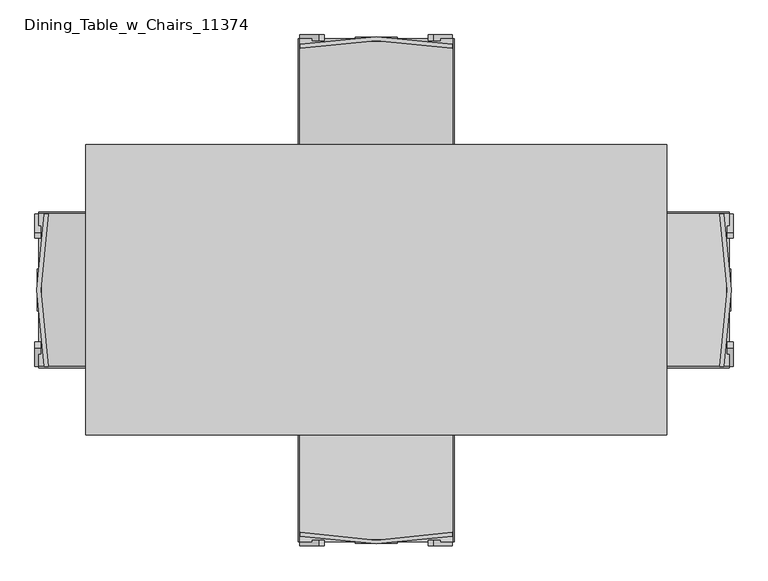
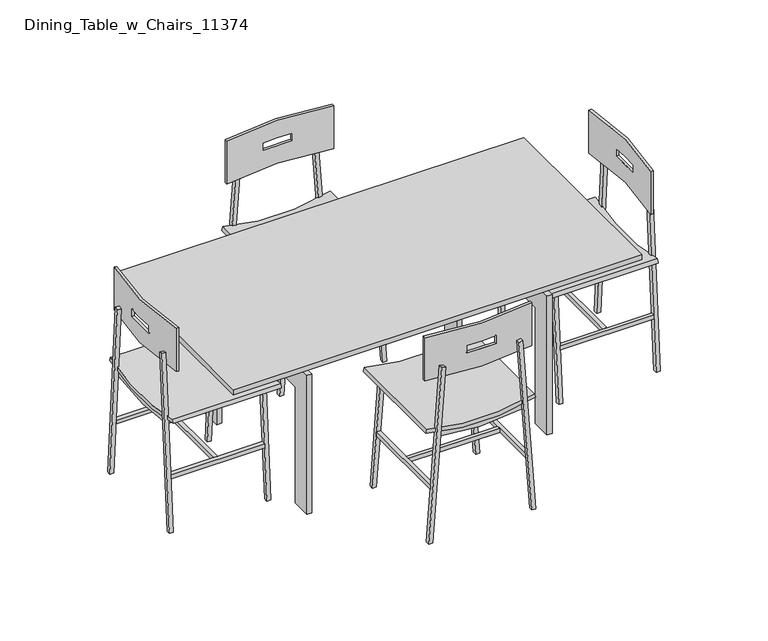
"""IFC4 building model written with IfcOpenShell, lengths in millimetres: furniture geometry, Dining_Table_w_Chairs_11374."""

from ifc_helpers import new_model, si_unit, point, frame, frame_2d, origin, place, context, project, spatial, polyline, circle_curve, trimmed, segment, composite_curve, outline, extrude, source, transform, mapped, element, save
from ifc_brep_helpers import plane_surface, cylinder_surface, revolved_surface, advanced_brep


def dining_table_w_chairs_11374_0cdfc61b(model_context):
    return source(origin(), model_context, "Body", "SolidModel", [
        extrude(outline(polyline([(780.7657667, 476.2110778), (780.7657667, -285.7889222), (-744.2342333, -285.7889222), (-744.2342333, 476.2110778), (780.7657667, 476.2110778)])), frame((0.0, 0.0, 609.8934749), z_axis=(0.0, 0.0, 1.0), x_axis=(1.0, 0.0, 0.0)), (0.0, 0.0, 1.0), 20.463567),
        extrude(outline(polyline([(425.4110778, 549.1807152), (425.4110778, 0.0), (349.2110778, 0.0), (349.2110778, 457.24037), (-158.7889222, 457.24037), (-158.7889222, 0.0), (-234.9889222, 0.0), (-234.9889222, 549.1807152), (425.4110778, 549.1807152)])), frame((-439.4342333, 0.0, 0.0), z_axis=(1.0, 0.0, 0.0), x_axis=(0.0, 1.0, 0.0)), (0.0, 0.0, 1.0), 19.05),
        extrude(outline(polyline([(425.4110778, 0.0), (349.2110778, 0.0), (349.2110778, 457.24037), (-158.7889222, 457.24037), (-158.7889222, 0.0), (-234.9889222, 0.0), (-234.9889222, 549.1807152), (425.4110778, 549.1807152), (425.4110778, 0.0)])), frame((456.9157667, 0.0, 0.0), z_axis=(1.0, 0.0, 0.0), x_axis=(0.0, 1.0, 0.0)), (0.0, 0.0, 1.0), 19.05),
        extrude(outline(polyline([(679.1657667, 297.7823857), (679.1657667, 272.3823857), (-642.6342333, 272.3823857), (-642.6342333, 297.7823857), (679.1657667, 297.7823857)])), frame((0.0, 0.0, 549.1807152), z_axis=(0.0, 0.0, 1.0), x_axis=(1.0, 0.0, 0.0)), (0.0, 0.0, 1.0), 60.7127597),
        extrude(outline(polyline([(679.1657667, -82.5889222), (679.1657667, -107.9889222), (-642.6342333, -107.9889222), (-642.6342333, -82.5889222), (679.1657667, -82.5889222)])), frame((0.0, 0.0, 549.1807152), z_axis=(0.0, 0.0, 1.0), x_axis=(1.0, 0.0, 0.0)), (0.0, 0.0, 1.0), 60.7127597),
        extrude(outline(composite_curve([segment(trimmed(circle_curve(frame_2d((1170.3570419, 17.9056041)), 750.0), [point((447.7280267, 218.6724002))], [point((447.7280267, -182.861192))], True, "CARTESIAN"), True, "CONTINUOUS"), segment(polyline([(447.7280267, -182.861192), (433.3268701, -187.0615294)]), True, "CONTINUOUS"), segment(trimmed(circle_curve(frame_2d((1170.3570419, 17.9056041)), 765.0), [point((433.3268701, -187.0615294))], [point((433.3268701, 222.8727375))], False, "CARTESIAN"), True, "CONTINUOUS"), segment(polyline([(433.3268701, 222.8727375), (447.7280267, 218.6724002)]), True, "CONTINUOUS")], self_intersect=False)), frame((0.0, 349.5931558, 0.0), z_axis=(0.0, 1.0, 0.0), x_axis=(0.0, 0.0, 1.0)), (0.0, 0.0, 1.0), 404.4405515),
        extrude(outline(polyline([(188.3951225, 567.5931558), (-151.5116757, 567.5931558), (-151.5116757, 582.5931558), (188.3951225, 582.5931558), (188.3951225, 567.5931558)])), frame((0.0, 0.0, 202.4578286), z_axis=(0.0, 0.0, 1.0), x_axis=(1.0, 0.0, 0.0)), (0.0, 0.0, 1.0), 15.0),
        extrude(outline(polyline([(203.3951225, 749.5931558), (203.3951225, 400.5931558), (188.3951225, 400.5931558), (188.3951225, 749.5931558), (203.3951225, 749.5931558)])), frame((0.0, 0.0, 202.4578286), z_axis=(0.0, 0.0, 1.0), x_axis=(1.0, 0.0, 0.0)), (0.0, 0.0, 1.0), 15.0),
        extrude(outline(polyline([(-152.6221887, 749.5931558), (-152.6221887, 400.5931558), (-167.6221887, 400.5931558), (-167.6221887, 749.5931558), (-152.6221887, 749.5931558)])), frame((0.0, 0.0, 202.4578286), z_axis=(0.0, 0.0, 1.0), x_axis=(1.0, 0.0, 0.0)), (0.0, 0.0, 1.0), 15.0),
        extrude(outline(polyline([(424.4138727, -151.781721), (0.0, -182.1199182), (0.0, -167.0816438), (421.1991529, -136.9732431), (424.4138727, -151.781721)])), frame((0.0, 385.5931558, 0.0), z_axis=(0.0, 1.0, 0.0), x_axis=(0.0, 0.0, 1.0)), (0.0, 0.0, 1.0), 15.0),
        extrude(outline(polyline([(424.4138727, 187.5929292), (421.1991529, 172.7844513), (0.0, 202.892852), (0.0, 217.9311264), (424.4138727, 187.5929292)])), frame((0.0, 385.5931558, 0.0), z_axis=(0.0, 1.0, 0.0), x_axis=(0.0, 0.0, 1.0)), (0.0, 0.0, 1.0), 15.0),
        extrude(outline(polyline([(680.7398074, 169.2700909), (677.5250876, 154.461613), (0.0, 202.892852), (0.0, 217.9311264), (680.7398074, 169.2700909)])), frame((0.0, 749.5931558, 0.0), z_axis=(0.0, 1.0, 0.0), x_axis=(0.0, 0.0, 1.0)), (0.0, 0.0, 1.0), 15.0),
        extrude(outline(polyline([(680.7398074, -133.4588828), (0.0, -182.1199182), (0.0, -167.0816438), (677.5250876, -118.6504049), (680.7398074, -133.4588828)])), frame((0.0, 749.5931558, 0.0), z_axis=(0.0, 1.0, 0.0), x_axis=(0.0, 0.0, 1.0)), (0.0, 0.0, 1.0), 15.0),
        advanced_brep(
        [(-182.0943959, 739.5931558, 800.3570419), (-182.0943959, 729.5931558, 800.3570419), (217.9056041, 729.5931558, 800.3570419), (217.9056041, 739.5931558, 800.3570419), (-182.0943959, 739.5931558, 630.3570419), (217.9056041, 739.5931558, 630.3570419), (217.9056041, 729.5931558, 630.3570419), (-182.0943959, 729.5931558, 630.3570419), (-37.0943959, 748.2797933, 730.3570419), (72.9056041, 748.2797933, 730.3570419), (72.9056041, 748.2797933, 700.3570419), (-37.0943959, 748.2797933, 700.3570419), (72.9056041, 758.0945192, 730.3570419), (-37.0943959, 758.0945192, 730.3570419), (-37.0943959, 758.0945192, 700.3570419), (72.9056041, 758.0945192, 700.3570419)],
        [
            (0, 1),
            (1, 2, circle_curve(frame((17.9056041, -250.4068442, 800.3570419), z_axis=(0.0, 0.0, -1.0), x_axis=(1.0, 0.0, 0.0)), 1000.19998)),
            (2, 3),
            (3, 0, circle_curve(frame((17.9056041, -250.4068442, 800.3570419), z_axis=(0.0, 0.0, 1.0), x_axis=(1.0, 0.0, 0.0)), 1010.0)),
            (4, 5, circle_curve(frame((17.9056041, -250.4068442, 630.3570419), z_axis=(0.0, 0.0, -1.0), x_axis=(1.0, 0.0, 0.0)), 1010.0)),
            (5, 6),
            (6, 7, circle_curve(frame((17.9056041, -250.4068442, 630.3570419), z_axis=(0.0, 0.0, 1.0), x_axis=(1.0, 0.0, 0.0)), 1000.19998)),
            (7, 4),
            (0, 4),
            (7, 1),
            (6, 2),
            (8, 9, circle_curve(frame((17.9056041, -250.4068442, 730.3570419), z_axis=(0.0, 0.0, -1.0), x_axis=(1.0, 0.0, 0.0)), 1000.19998)),
            (9, 10),
            (10, 11, circle_curve(frame((17.9056041, -250.4068442, 700.3570419), z_axis=(0.0, 0.0, 1.0), x_axis=(1.0, 0.0, 0.0)), 1000.19998)),
            (11, 8),
            (5, 3),
            (12, 13, circle_curve(frame((17.9056041, -250.4068442, 730.3570419), z_axis=(0.0, 0.0, 1.0), x_axis=(1.0, 0.0, 0.0)), 1010.0)),
            (13, 14),
            (14, 15, circle_curve(frame((17.9056041, -250.4068442, 700.3570419), z_axis=(0.0, 0.0, -1.0), x_axis=(1.0, 0.0, 0.0)), 1010.0)),
            (15, 12),
            (12, 9),
            (8, 13),
            (11, 14),
            (10, 15),
        ],
        [
            plane_surface(frame((-182.0943959, 739.5931558, 800.3570419), z_axis=(0.0, 0.0, 1.0), x_axis=(0.0, -1.0, 0.0))),
            plane_surface(frame((-182.0943959, 739.5931558, 630.3570419), z_axis=(0.0, 0.0, -1.0), x_axis=(0.0, 1.0, 0.0))),
            plane_surface(frame((-182.0943959, 739.5931558, 800.3570419), z_axis=(-1.0, 0.0, 0.0), x_axis=(0.0, 0.0, -1.0))),
            revolved_surface(polyline([(1018.1055841, -250.4068442, 630.3570419), (1018.1055841, -250.4068442, 800.3570419)]), (17.9056041, -250.4068442, 630.3570419), (0.0, 0.0, -1.0)),
            plane_surface(frame((217.9056041, 729.5931558, 800.3570419), z_axis=(1.0, 0.0, 0.0), x_axis=(0.0, 0.0, -1.0))),
            cylinder_surface(frame((17.9056041, -250.4068442, 630.3570419), z_axis=(0.0, 0.0, 1.0), x_axis=(1.0, 0.0, 0.0)), 1010.0),
            plane_surface(frame((72.9056041, 695.0477456, 730.3570419), z_axis=(0.0, 0.0, -1.0), x_axis=(0.0, 1.0, 0.0))),
            plane_surface(frame((-37.0943959, 695.0477456, 730.3570419), z_axis=(1.0, 0.0, 0.0), x_axis=(0.0, 1.0, 0.0))),
            plane_surface(frame((-37.0943959, 695.0477456, 700.3570419), z_axis=(0.0, 0.0, 1.0), x_axis=(0.0, 1.0, 0.0))),
            plane_surface(frame((72.9056041, 695.0477456, 700.3570419), z_axis=(-1.0, 0.0, 0.0), x_axis=(0.0, 1.0, 0.0))),
        ],
        [
            (0, [[1, 2, 3, 4]]),
            (1, [[5, 6, 7, 8]]),
            (2, [[-1, 9, -8, 10]]),
            (3, [[-2, -10, -7, 11], [12, 13, 14, 15]]),
            (4, [[-3, -11, -6, 16]]),
            (5, [[-4, -16, -5, -9], [17, 18, 19, 20]]),
            (6, [[21, -12, 22, -17]]),
            (7, [[-22, -15, 23, -18]]),
            (8, [[-23, -14, 24, -19]]),
            (9, [[-21, -20, -24, -13]]),
        ],
    ),
        extrude(outline(composite_curve([segment(polyline([(295.2420652, 447.7247508), (299.4424026, 433.3235941)]), True, "CONTINUOUS"), segment(trimmed(circle_curve(frame_2d((94.4752691, 1170.353766)), 765.0), [point((299.4424026, 433.3235941))], [point((-110.4918643, 433.3235941))], False, "CARTESIAN"), True, "CONTINUOUS"), segment(polyline([(-110.4918643, 433.3235941), (-106.291527, 447.7247508)]), True, "CONTINUOUS"), segment(trimmed(circle_curve(frame_2d((94.4752691, 1170.353766)), 750.0), [point((-106.291527, 447.7247508))], [point((295.2420652, 447.7247508))], True, "CARTESIAN"), True, "CONTINUOUS")], self_intersect=False)), frame((-867.0747848, 0.0, 0.0), z_axis=(1.0, 0.0, 0.0), x_axis=(0.0, 1.0, 0.0)), (0.0, 0.0, 1.0), 404.4405515),
        extrude(outline(polyline([(-680.6342333, 264.9647875), (-680.6342333, -74.9420106), (-695.6342333, -74.9420106), (-695.6342333, 264.9647875), (-680.6342333, 264.9647875)])), frame((0.0, 0.0, 202.4545527), z_axis=(0.0, 0.0, 1.0), x_axis=(1.0, 0.0, 0.0)), (0.0, 0.0, 1.0), 15.0),
        extrude(outline(polyline([(-862.6342333, 279.9647875), (-513.6342333, 279.9647875), (-513.6342333, 264.9647875), (-862.6342333, 264.9647875), (-862.6342333, 279.9647875)])), frame((0.0, 0.0, 202.4545527), z_axis=(0.0, 0.0, 1.0), x_axis=(1.0, 0.0, 0.0)), (0.0, 0.0, 1.0), 15.0),
        extrude(outline(polyline([(-862.6342333, -76.0525236), (-513.6342333, -76.0525236), (-513.6342333, -91.0525236), (-862.6342333, -91.0525236), (-862.6342333, -76.0525236)])), frame((0.0, 0.0, 202.4545527), z_axis=(0.0, 0.0, 1.0), x_axis=(1.0, 0.0, 0.0)), (0.0, 0.0, 1.0), 15.0),
        extrude(outline(polyline([(-75.212056, 424.4105968), (-60.4035781, 421.195877), (-90.5119788, -0.0032759), (-105.5502532, -0.0032759), (-75.212056, 424.4105968)])), frame((-513.6342333, 0.0, 0.0), z_axis=(1.0, 0.0, 0.0), x_axis=(0.0, 1.0, 0.0)), (0.0, 0.0, 1.0), 15.0),
        extrude(outline(polyline([(264.1625942, 424.4105968), (294.5007914, -0.0032759), (279.462517, -0.0032759), (249.3541163, 421.195877), (264.1625942, 424.4105968)])), frame((-513.6342333, 0.0, 0.0), z_axis=(1.0, 0.0, 0.0), x_axis=(0.0, 1.0, 0.0)), (0.0, 0.0, 1.0), 15.0),
        extrude(outline(polyline([(245.839756, 680.7365315), (294.5007914, -0.0032759), (279.462517, -0.0032759), (231.0312781, 677.5218117), (245.839756, 680.7365315)])), frame((-877.6342333, 0.0, 0.0), z_axis=(1.0, 0.0, 0.0), x_axis=(0.0, 1.0, 0.0)), (0.0, 0.0, 1.0), 15.0),
        extrude(outline(polyline([(-56.8892177, 680.7365315), (-42.0807398, 677.5218117), (-90.5119788, -0.0032759), (-105.5502532, -0.0032759), (-56.8892177, 680.7365315)])), frame((-877.6342333, 0.0, 0.0), z_axis=(1.0, 0.0, 0.0), x_axis=(0.0, 1.0, 0.0)), (0.0, 0.0, 1.0), 15.0),
        advanced_brep(
        [(-852.6342333, -105.5247309, 800.353766), (-842.6342333, -105.5247309, 800.353766), (-842.6342333, 294.4752691, 800.353766), (-852.6342333, 294.4752691, 800.353766), (-852.6342333, -105.5247309, 630.353766), (-852.6342333, 294.4752691, 630.353766), (-842.6342333, 294.4752691, 630.353766), (-842.6342333, -105.5247309, 630.353766), (-861.3208709, 39.4752691, 730.353766), (-861.3208709, 149.4752691, 730.353766), (-861.3208709, 149.4752691, 700.353766), (-861.3208709, 39.4752691, 700.353766), (-871.1355967, 149.4752691, 730.353766), (-871.1355967, 39.4752691, 730.353766), (-871.1355967, 39.4752691, 700.353766), (-871.1355967, 149.4752691, 700.353766)],
        [
            (0, 1),
            (1, 2, circle_curve(frame((137.3657667, 94.4752691, 800.353766), z_axis=(0.0, 0.0, -1.0), x_axis=(0.0, 1.0, 0.0)), 1000.19998)),
            (2, 3),
            (3, 0, circle_curve(frame((137.3657667, 94.4752691, 800.353766), z_axis=(0.0, 0.0, 1.0), x_axis=(0.0, 1.0, 0.0)), 1010.0)),
            (4, 5, circle_curve(frame((137.3657667, 94.4752691, 630.353766), z_axis=(0.0, 0.0, -1.0), x_axis=(0.0, 1.0, 0.0)), 1010.0)),
            (5, 6),
            (6, 7, circle_curve(frame((137.3657667, 94.4752691, 630.353766), z_axis=(0.0, 0.0, 1.0), x_axis=(0.0, 1.0, 0.0)), 1000.19998)),
            (7, 4),
            (0, 4),
            (7, 1),
            (6, 2),
            (8, 9, circle_curve(frame((137.3657667, 94.4752691, 730.353766), z_axis=(0.0, 0.0, -1.0), x_axis=(0.0, 1.0, 0.0)), 1000.19998)),
            (9, 10),
            (10, 11, circle_curve(frame((137.3657667, 94.4752691, 700.353766), z_axis=(0.0, 0.0, 1.0), x_axis=(0.0, 1.0, 0.0)), 1000.19998)),
            (11, 8),
            (5, 3),
            (12, 13, circle_curve(frame((137.3657667, 94.4752691, 730.353766), z_axis=(0.0, 0.0, 1.0), x_axis=(0.0, 1.0, 0.0)), 1010.0)),
            (13, 14),
            (14, 15, circle_curve(frame((137.3657667, 94.4752691, 700.353766), z_axis=(0.0, 0.0, -1.0), x_axis=(0.0, 1.0, 0.0)), 1010.0)),
            (15, 12),
            (12, 9),
            (8, 13),
            (11, 14),
            (10, 15),
        ],
        [
            plane_surface(frame((-852.6342333, -105.5247309, 800.353766), z_axis=(0.0, 0.0, 1.0), x_axis=(1.0, 0.0, 0.0))),
            plane_surface(frame((-852.6342333, -105.5247309, 630.353766), z_axis=(0.0, 0.0, -1.0), x_axis=(-1.0, 0.0, 0.0))),
            plane_surface(frame((-852.6342333, -105.5247309, 800.353766), z_axis=(0.0, -1.0, 0.0), x_axis=(0.0, 0.0, -1.0))),
            revolved_surface(polyline([(137.3657667, 1094.6752491, 630.353766), (137.3657667, 1094.6752491, 800.353766)]), (137.3657667, 94.4752691, 630.353766), (0.0, 0.0, -1.0)),
            plane_surface(frame((-842.6342333, 294.4752691, 800.353766), z_axis=(0.0, 1.0, 0.0), x_axis=(0.0, 0.0, -1.0))),
            cylinder_surface(frame((137.3657667, 94.4752691, 630.353766), z_axis=(0.0, 0.0, 1.0), x_axis=(0.0, 1.0, 0.0)), 1010.0),
            plane_surface(frame((-808.0888232, 149.4752691, 730.353766), z_axis=(0.0, 0.0, -1.0), x_axis=(-1.0, 0.0, 0.0))),
            plane_surface(frame((-808.0888232, 39.4752691, 730.353766), z_axis=(0.0, 1.0, 0.0), x_axis=(-1.0, 0.0, 0.0))),
            plane_surface(frame((-808.0888232, 39.4752691, 700.353766), z_axis=(0.0, 0.0, 1.0), x_axis=(-1.0, 0.0, 0.0))),
            plane_surface(frame((-808.0888232, 149.4752691, 700.353766), z_axis=(0.0, -1.0, 0.0), x_axis=(-1.0, 0.0, 0.0))),
        ],
        [
            (0, [[1, 2, 3, 4]]),
            (1, [[5, 6, 7, 8]]),
            (2, [[-1, 9, -8, 10]]),
            (3, [[-2, -10, -7, 11], [12, 13, 14, 15]]),
            (4, [[-3, -11, -6, 16]]),
            (5, [[-4, -16, -5, -9], [17, 18, 19, 20]]),
            (6, [[21, -12, 22, -17]]),
            (7, [[-22, -15, 23, -18]]),
            (8, [[-23, -14, 24, -19]]),
            (9, [[-21, -20, -24, -13]]),
        ],
    ),
        extrude(outline(composite_curve([segment(trimmed(circle_curve(frame_2d((94.4752691, 1170.3570419)), 750.0), [point((-106.291527, 447.7280267))], [point((295.2420652, 447.7280267))], True, "CARTESIAN"), True, "CONTINUOUS"), segment(polyline([(295.2420652, 447.7280267), (299.4424026, 433.3268701)]), True, "CONTINUOUS"), segment(trimmed(circle_curve(frame_2d((94.4752691, 1170.3570419)), 765.0), [point((299.4424026, 433.3268701))], [point((-110.4918643, 433.3268701))], False, "CARTESIAN"), True, "CONTINUOUS"), segment(polyline([(-110.4918643, 433.3268701), (-106.291527, 447.7280267)]), True, "CONTINUOUS")], self_intersect=False)), frame((539.2330291, 0.0, 0.0), z_axis=(1.0, 0.0, 0.0), x_axis=(0.0, 1.0, 0.0)), (0.0, 0.0, 1.0), 404.4405515),
        extrude(outline(polyline([(757.2330291, -76.0142493), (757.2330291, 263.8925489), (772.2330291, 263.8925489), (772.2330291, -76.0142493), (757.2330291, -76.0142493)])), frame((0.0, 0.0, 202.4578286), z_axis=(0.0, 0.0, 1.0), x_axis=(1.0, 0.0, 0.0)), (0.0, 0.0, 1.0), 15.0),
        extrude(outline(polyline([(939.2330291, -91.0142493), (590.2330291, -91.0142493), (590.2330291, -76.0142493), (939.2330291, -76.0142493), (939.2330291, -91.0142493)])), frame((0.0, 0.0, 202.4578286), z_axis=(0.0, 0.0, 1.0), x_axis=(1.0, 0.0, 0.0)), (0.0, 0.0, 1.0), 15.0),
        extrude(outline(polyline([(939.2330291, 265.0030619), (590.2330291, 265.0030619), (590.2330291, 280.0030619), (939.2330291, 280.0030619), (939.2330291, 265.0030619)])), frame((0.0, 0.0, 202.4578286), z_axis=(0.0, 0.0, 1.0), x_axis=(1.0, 0.0, 0.0)), (0.0, 0.0, 1.0), 15.0),
        extrude(outline(polyline([(264.1625942, 424.4138727), (294.5007914, 0.0), (279.462517, 0.0), (249.3541163, 421.1991529), (264.1625942, 424.4138727)])), frame((575.2330291, 0.0, 0.0), z_axis=(1.0, 0.0, 0.0), x_axis=(0.0, 1.0, 0.0)), (0.0, 0.0, 1.0), 15.0),
        extrude(outline(polyline([(-75.212056, 424.4138727), (-60.4035781, 421.1991529), (-90.5119788, 0.0), (-105.5502532, 0.0), (-75.212056, 424.4138727)])), frame((575.2330291, 0.0, 0.0), z_axis=(1.0, 0.0, 0.0), x_axis=(0.0, 1.0, 0.0)), (0.0, 0.0, 1.0), 15.0),
        extrude(outline(polyline([(-56.8892177, 680.7398074), (-42.0807398, 677.5250876), (-90.5119788, 0.0), (-105.5502532, 0.0), (-56.8892177, 680.7398074)])), frame((939.2330291, 0.0, 0.0), z_axis=(1.0, 0.0, 0.0), x_axis=(0.0, 1.0, 0.0)), (0.0, 0.0, 1.0), 15.0),
        extrude(outline(polyline([(245.839756, 680.7398074), (294.5007914, 0.0), (279.462517, 0.0), (231.0312781, 677.5250876), (245.839756, 680.7398074)])), frame((939.2330291, 0.0, 0.0), z_axis=(1.0, 0.0, 0.0), x_axis=(0.0, 1.0, 0.0)), (0.0, 0.0, 1.0), 15.0),
        advanced_brep(
        [(929.2330291, 294.4752691, 800.3570419), (919.2330291, 294.4752691, 800.3570419), (919.2330291, -105.5247309, 800.3570419), (929.2330291, -105.5247309, 800.3570419), (929.2330291, 294.4752691, 630.3570419), (929.2330291, -105.5247309, 630.3570419), (919.2330291, -105.5247309, 630.3570419), (919.2330291, 294.4752691, 630.3570419), (937.9196666, 149.4752691, 730.3570419), (937.9196666, 39.4752691, 730.3570419), (937.9196666, 39.4752691, 700.3570419), (937.9196666, 149.4752691, 700.3570419), (947.7343925, 39.4752691, 730.3570419), (947.7343925, 149.4752691, 730.3570419), (947.7343925, 149.4752691, 700.3570419), (947.7343925, 39.4752691, 700.3570419)],
        [
            (0, 1),
            (1, 2, circle_curve(frame((-60.7669709, 94.4752691, 800.3570419), z_axis=(0.0, 0.0, -1.0), x_axis=(0.0, -1.0, 0.0)), 1000.19998)),
            (2, 3),
            (3, 0, circle_curve(frame((-60.7669709, 94.4752691, 800.3570419), z_axis=(0.0, 0.0, 1.0), x_axis=(0.0, -1.0, 0.0)), 1010.0)),
            (4, 5, circle_curve(frame((-60.7669709, 94.4752691, 630.3570419), z_axis=(0.0, 0.0, -1.0), x_axis=(0.0, -1.0, 0.0)), 1010.0)),
            (5, 6),
            (6, 7, circle_curve(frame((-60.7669709, 94.4752691, 630.3570419), z_axis=(0.0, 0.0, 1.0), x_axis=(0.0, -1.0, 0.0)), 1000.19998)),
            (7, 4),
            (0, 4),
            (7, 1),
            (6, 2),
            (8, 9, circle_curve(frame((-60.7669709, 94.4752691, 730.3570419), z_axis=(0.0, 0.0, -1.0), x_axis=(0.0, -1.0, 0.0)), 1000.19998)),
            (9, 10),
            (10, 11, circle_curve(frame((-60.7669709, 94.4752691, 700.3570419), z_axis=(0.0, 0.0, 1.0), x_axis=(0.0, -1.0, 0.0)), 1000.19998)),
            (11, 8),
            (5, 3),
            (12, 13, circle_curve(frame((-60.7669709, 94.4752691, 730.3570419), z_axis=(0.0, 0.0, 1.0), x_axis=(0.0, -1.0, 0.0)), 1010.0)),
            (13, 14),
            (14, 15, circle_curve(frame((-60.7669709, 94.4752691, 700.3570419), z_axis=(0.0, 0.0, -1.0), x_axis=(0.0, -1.0, 0.0)), 1010.0)),
            (15, 12),
            (12, 9),
            (8, 13),
            (11, 14),
            (10, 15),
        ],
        [
            plane_surface(frame((929.2330291, 294.4752691, 800.3570419), z_axis=(0.0, 0.0, 1.0), x_axis=(-1.0, 0.0, 0.0))),
            plane_surface(frame((929.2330291, 294.4752691, 630.3570419), z_axis=(0.0, 0.0, -1.0), x_axis=(1.0, 0.0, 0.0))),
            plane_surface(frame((929.2330291, 294.4752691, 800.3570419), z_axis=(0.0, 1.0, 0.0), x_axis=(0.0, 0.0, -1.0))),
            revolved_surface(polyline([(-60.7669709, -905.7247109, 630.3570419), (-60.7669709, -905.7247109, 800.3570419)]), (-60.7669709, 94.4752691, 630.3570419), (0.0, 0.0, -1.0)),
            plane_surface(frame((919.2330291, -105.5247309, 800.3570419), z_axis=(0.0, -1.0, 0.0), x_axis=(0.0, 0.0, -1.0))),
            cylinder_surface(frame((-60.7669709, 94.4752691, 630.3570419), z_axis=(0.0, 0.0, 1.0), x_axis=(0.0, -1.0, 0.0)), 1010.0),
            plane_surface(frame((884.6876189, 39.4752691, 730.3570419), z_axis=(0.0, 0.0, -1.0), x_axis=(1.0, 0.0, 0.0))),
            plane_surface(frame((884.6876189, 149.4752691, 730.3570419), z_axis=(0.0, -1.0, 0.0), x_axis=(1.0, 0.0, 0.0))),
            plane_surface(frame((884.6876189, 149.4752691, 700.3570419), z_axis=(0.0, 0.0, 1.0), x_axis=(1.0, 0.0, 0.0))),
            plane_surface(frame((884.6876189, 39.4752691, 700.3570419), z_axis=(0.0, 1.0, 0.0), x_axis=(1.0, 0.0, 0.0))),
        ],
        [
            (0, [[1, 2, 3, 4]]),
            (1, [[5, 6, 7, 8]]),
            (2, [[-1, 9, -8, 10]]),
            (3, [[-2, -10, -7, 11], [12, 13, 14, 15]]),
            (4, [[-3, -11, -6, 16]]),
            (5, [[-4, -16, -5, -9], [17, 18, 19, 20]]),
            (6, [[21, -12, 22, -17]]),
            (7, [[-22, -15, 23, -18]]),
            (8, [[-23, -14, 24, -19]]),
            (9, [[-21, -20, -24, -13]]),
        ],
    ),
        extrude(outline(composite_curve([segment(polyline([(447.7280267, -182.861192), (433.3268701, -187.0615294)]), True, "CONTINUOUS"), segment(trimmed(circle_curve(frame_2d((1170.3570419, 17.9056041)), 765.0), [point((433.3268701, -187.0615294))], [point((433.3268701, 222.8727375))], False, "CARTESIAN"), True, "CONTINUOUS"), segment(polyline([(433.3268701, 222.8727375), (447.7280267, 218.6724002)]), True, "CONTINUOUS"), segment(trimmed(circle_curve(frame_2d((1170.3570419, 17.9056041)), 750.0), [point((447.7280267, 218.6724002))], [point((447.7280267, -182.861192))], True, "CARTESIAN"), True, "CONTINUOUS")], self_intersect=False)), frame((0.0, -566.7146581, 0.0), z_axis=(0.0, 1.0, 0.0), x_axis=(0.0, 0.0, 1.0)), (0.0, 0.0, 1.0), 404.4405515),
        extrude(outline(polyline([(-152.5839143, -380.2741066), (187.3228838, -380.2741066), (187.3228838, -395.2741066), (-152.5839143, -395.2741066), (-152.5839143, -380.2741066)])), frame((0.0, 0.0, 202.4578286), z_axis=(0.0, 0.0, 1.0), x_axis=(1.0, 0.0, 0.0)), (0.0, 0.0, 1.0), 15.0),
        extrude(outline(polyline([(-167.5839143, -562.2741066), (-167.5839143, -213.2741066), (-152.5839143, -213.2741066), (-152.5839143, -562.2741066), (-167.5839143, -562.2741066)])), frame((0.0, 0.0, 202.4578286), z_axis=(0.0, 0.0, 1.0), x_axis=(1.0, 0.0, 0.0)), (0.0, 0.0, 1.0), 15.0),
        extrude(outline(polyline([(188.4333968, -562.2741066), (188.4333968, -213.2741066), (203.4333968, -213.2741066), (203.4333968, -562.2741066), (188.4333968, -562.2741066)])), frame((0.0, 0.0, 202.4578286), z_axis=(0.0, 0.0, 1.0), x_axis=(1.0, 0.0, 0.0)), (0.0, 0.0, 1.0), 15.0),
        extrude(outline(polyline([(424.4138727, 187.5929292), (421.1991529, 172.7844513), (0.0, 202.892852), (0.0, 217.9311264), (424.4138727, 187.5929292)])), frame((0.0, -213.2741066, 0.0), z_axis=(0.0, 1.0, 0.0), x_axis=(0.0, 0.0, 1.0)), (0.0, 0.0, 1.0), 15.0),
        extrude(outline(polyline([(424.4138727, -151.781721), (0.0, -182.1199182), (0.0, -167.0816438), (421.1991529, -136.9732431), (424.4138727, -151.781721)])), frame((0.0, -213.2741066, 0.0), z_axis=(0.0, 1.0, 0.0), x_axis=(0.0, 0.0, 1.0)), (0.0, 0.0, 1.0), 15.0),
        extrude(outline(polyline([(680.7398074, -133.4588828), (0.0, -182.1199182), (0.0, -167.0816438), (677.5250876, -118.6504049), (680.7398074, -133.4588828)])), frame((0.0, -577.2741066, 0.0), z_axis=(0.0, 1.0, 0.0), x_axis=(0.0, 0.0, 1.0)), (0.0, 0.0, 1.0), 15.0),
        extrude(outline(polyline([(680.7398074, 169.2700909), (677.5250876, 154.461613), (0.0, 202.892852), (0.0, 217.9311264), (680.7398074, 169.2700909)])), frame((0.0, -577.2741066, 0.0), z_axis=(0.0, 1.0, 0.0), x_axis=(0.0, 0.0, 1.0)), (0.0, 0.0, 1.0), 15.0),
        advanced_brep(
        [(217.9056041, -552.2741066, 800.3570419), (217.9056041, -542.2741066, 800.3570419), (-182.0943959, -542.2741066, 800.3570419), (-182.0943959, -552.2741066, 800.3570419), (217.9056041, -552.2741066, 630.3570419), (-182.0943959, -552.2741066, 630.3570419), (-182.0943959, -542.2741066, 630.3570419), (217.9056041, -542.2741066, 630.3570419), (72.9056041, -560.9607442, 730.3570419), (-37.0943959, -560.9607442, 730.3570419), (-37.0943959, -560.9607442, 700.3570419), (72.9056041, -560.9607442, 700.3570419), (-37.0943959, -570.77547, 730.3570419), (72.9056041, -570.77547, 730.3570419), (72.9056041, -570.77547, 700.3570419), (-37.0943959, -570.77547, 700.3570419)],
        [
            (0, 1),
            (1, 2, circle_curve(frame((17.9056041, 437.7258934, 800.3570419), z_axis=(0.0, 0.0, -1.0), x_axis=(-1.0, 0.0, 0.0)), 1000.19998)),
            (2, 3),
            (3, 0, circle_curve(frame((17.9056041, 437.7258934, 800.3570419), z_axis=(0.0, 0.0, 1.0), x_axis=(-1.0, 0.0, 0.0)), 1010.0)),
            (4, 5, circle_curve(frame((17.9056041, 437.7258934, 630.3570419), z_axis=(0.0, 0.0, -1.0), x_axis=(-1.0, 0.0, 0.0)), 1010.0)),
            (5, 6),
            (6, 7, circle_curve(frame((17.9056041, 437.7258934, 630.3570419), z_axis=(0.0, 0.0, 1.0), x_axis=(-1.0, 0.0, 0.0)), 1000.19998)),
            (7, 4),
            (0, 4),
            (7, 1),
            (6, 2),
            (8, 9, circle_curve(frame((17.9056041, 437.7258934, 730.3570419), z_axis=(0.0, 0.0, -1.0), x_axis=(-1.0, 0.0, 0.0)), 1000.19998)),
            (9, 10),
            (10, 11, circle_curve(frame((17.9056041, 437.7258934, 700.3570419), z_axis=(0.0, 0.0, 1.0), x_axis=(-1.0, 0.0, 0.0)), 1000.19998)),
            (11, 8),
            (5, 3),
            (12, 13, circle_curve(frame((17.9056041, 437.7258934, 730.3570419), z_axis=(0.0, 0.0, 1.0), x_axis=(-1.0, 0.0, 0.0)), 1010.0)),
            (13, 14),
            (14, 15, circle_curve(frame((17.9056041, 437.7258934, 700.3570419), z_axis=(0.0, 0.0, -1.0), x_axis=(-1.0, 0.0, 0.0)), 1010.0)),
            (15, 12),
            (12, 9),
            (8, 13),
            (11, 14),
            (10, 15),
        ],
        [
            plane_surface(frame((217.9056041, -552.2741066, 800.3570419), z_axis=(0.0, 0.0, 1.0), x_axis=(0.0, 1.0, 0.0))),
            plane_surface(frame((217.9056041, -552.2741066, 630.3570419), z_axis=(0.0, 0.0, -1.0), x_axis=(0.0, -1.0, 0.0))),
            plane_surface(frame((217.9056041, -552.2741066, 800.3570419), z_axis=(1.0, 0.0, 0.0), x_axis=(0.0, 0.0, -1.0))),
            revolved_surface(polyline([(-982.2943759, 437.7258934, 630.3570419), (-982.2943759, 437.7258934, 800.3570419)]), (17.9056041, 437.7258934, 630.3570419), (0.0, 0.0, -1.0)),
            plane_surface(frame((-182.0943959, -542.2741066, 800.3570419), z_axis=(-1.0, 0.0, 0.0), x_axis=(0.0, 0.0, -1.0))),
            cylinder_surface(frame((17.9056041, 437.7258934, 630.3570419), z_axis=(0.0, 0.0, 1.0), x_axis=(-1.0, 0.0, 0.0)), 1010.0),
            plane_surface(frame((-37.0943959, -507.7286965, 730.3570419), z_axis=(0.0, 0.0, -1.0), x_axis=(0.0, -1.0, 0.0))),
            plane_surface(frame((72.9056041, -507.7286965, 730.3570419), z_axis=(-1.0, 0.0, 0.0), x_axis=(0.0, -1.0, 0.0))),
            plane_surface(frame((72.9056041, -507.7286965, 700.3570419), z_axis=(0.0, 0.0, 1.0), x_axis=(0.0, -1.0, 0.0))),
            plane_surface(frame((-37.0943959, -507.7286965, 700.3570419), z_axis=(1.0, 0.0, 0.0), x_axis=(0.0, -1.0, 0.0))),
        ],
        [
            (0, [[1, 2, 3, 4]]),
            (1, [[5, 6, 7, 8]]),
            (2, [[-1, 9, -8, 10]]),
            (3, [[-2, -10, -7, 11], [12, 13, 14, 15]]),
            (4, [[-3, -11, -6, 16]]),
            (5, [[-4, -16, -5, -9], [17, 18, 19, 20]]),
            (6, [[21, -12, 22, -17]]),
            (7, [[-22, -15, 23, -18]]),
            (8, [[-23, -14, 24, -19]]),
            (9, [[-21, -20, -24, -13]]),
        ],
    ),
        extrude(outline(composite_curve([segment(trimmed(circle_curve(frame_2d((1170.3570419, 17.9056041)), 765.0), [point((421.1991529, 172.7844513))], [point((421.497943, -138.4115413))], True, "CARTESIAN"), True, "CONTINUOUS"), segment(polyline([(421.497943, -138.4115413), (401.0781913, -138.4115413)]), True, "CONTINUOUS"), segment(trimmed(circle_curve(frame_2d((1170.3570419, 17.9056041)), 785.0), [point((401.0781913, -138.4115413))], [point((401.0781913, 174.2227495))], False, "CARTESIAN"), True, "CONTINUOUS"), segment(polyline([(401.0781913, 174.2227495), (421.1991529, 172.7844513)]), True, "CONTINUOUS")], self_intersect=False)), frame((0.0, 385.5931558, 0.0), z_axis=(0.0, 1.0, 0.0), x_axis=(0.0, 0.0, 1.0)), (0.0, 0.0, 1.0), 364.0),
        extrude(outline(composite_curve([segment(polyline([(249.3541163, 421.195877), (250.7924145, 401.0749153)]), True, "CONTINUOUS"), segment(trimmed(circle_curve(frame_2d((94.4752691, 1170.353766)), 785.0), [point((250.7924145, 401.0749153))], [point((-61.8418763, 401.0749153))], False, "CARTESIAN"), True, "CONTINUOUS"), segment(polyline([(-61.8418763, 401.0749153), (-61.8418763, 421.494667)]), True, "CONTINUOUS"), segment(trimmed(circle_curve(frame_2d((94.4752691, 1170.353766)), 765.0), [point((-61.8418763, 421.494667))], [point((249.3541163, 421.195877))], True, "CARTESIAN"), True, "CONTINUOUS")], self_intersect=False)), frame((-862.6342333, 0.0, 0.0), z_axis=(1.0, 0.0, 0.0), x_axis=(0.0, 1.0, 0.0)), (0.0, 0.0, 1.0), 364.0),
        extrude(outline(composite_curve([segment(trimmed(circle_curve(frame_2d((94.4752691, 1170.3570419)), 765.0), [point((-60.4035781, 421.1991529))], [point((250.7924145, 421.497943))], True, "CARTESIAN"), True, "CONTINUOUS"), segment(polyline([(250.7924145, 421.497943), (250.7924145, 401.0781913)]), True, "CONTINUOUS"), segment(trimmed(circle_curve(frame_2d((94.4752691, 1170.3570419)), 785.0), [point((250.7924145, 401.0781913))], [point((-61.8418763, 401.0781913))], False, "CARTESIAN"), True, "CONTINUOUS"), segment(polyline([(-61.8418763, 401.0781913), (-60.4035781, 421.1991529)]), True, "CONTINUOUS")], self_intersect=False)), frame((575.2330291, 0.0, 0.0), z_axis=(1.0, 0.0, 0.0), x_axis=(0.0, 1.0, 0.0)), (0.0, 0.0, 1.0), 364.0),
        extrude(outline(composite_curve([segment(polyline([(421.1991529, -136.9732431), (401.0781912, -138.4115413)]), True, "CONTINUOUS"), segment(trimmed(circle_curve(frame_2d((1170.3570419, 17.9056041)), 785.0), [point((401.0781912, -138.4115413))], [point((401.0781913, 174.2227495))], False, "CARTESIAN"), True, "CONTINUOUS"), segment(polyline([(401.0781913, 174.2227495), (421.497943, 174.2227495)]), True, "CONTINUOUS"), segment(trimmed(circle_curve(frame_2d((1170.3570419, 17.9056041)), 765.0), [point((421.497943, 174.2227495))], [point((421.1991529, -136.9732431))], True, "CARTESIAN"), True, "CONTINUOUS")], self_intersect=False)), frame((0.0, -562.2741066, 0.0), z_axis=(0.0, 1.0, 0.0), x_axis=(0.0, 0.0, 1.0)), (0.0, 0.0, 1.0), 364.0),
    ])


if __name__ == "__main__":
    model = new_model("IFC4")
    model_context = context("Model", 3, world=origin())
    ifc_project = project(units=[si_unit("LENGTHUNIT", "METRE", prefix="MILLI")], contexts=[model_context])
    site = spatial("IfcSite", under=ifc_project)
    building = spatial("IfcBuilding", under=site)
    placement = place(None, origin())
    dining_table_w_chairs_11374_shape = dining_table_w_chairs_11374_0cdfc61b(model_context)
    element("IfcFurniture", 1, ObjectType="Dining_Table_w_Chairs_11374", at=placement, inside=building, context=model_context, shape_type="MappedRepresentation", body=[
        mapped(dining_table_w_chairs_11374_shape, transform((0.0, 0.0, 0.0), x_axis=(1.0, 0.0, 0.0), y_axis=(0.0, 1.0, 0.0), z_axis=(0.0, 0.0, 1.0))),
    ])
    save(model, "model.ifc")

# Revit data of these elements
# Type "Dining_Table_w_Chairs_11374"
#   Default Elevation = 0
#   Assembly Code = ""
